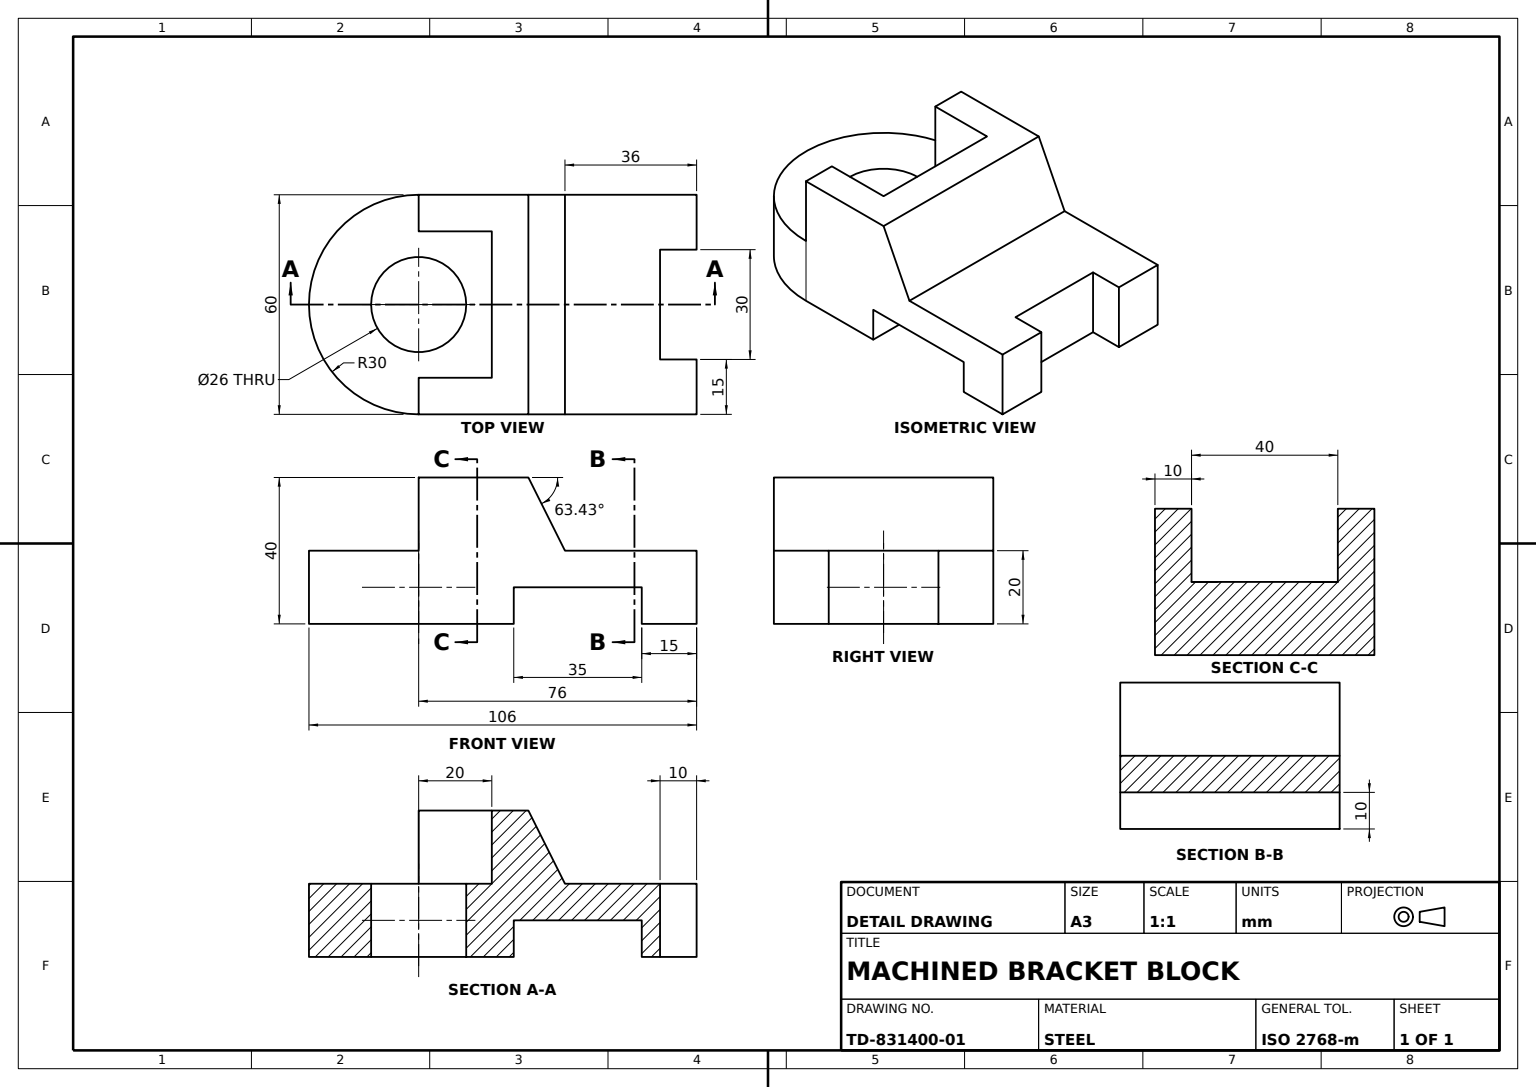
SolidWorks part; units mm, degrees
material "Plain Carbon Steel"
ref_plane "Front Plane" through (0, 0, 0) normal (0, 0, 1) x (1, 0, 0)
ref_plane "Top Plane" through (0, 0, 0) normal (0, 1, 0) x (1, 0, 0)
ref_plane "Right Plane" through (0, 0, 0) normal (1, 0, 0) x (0, 0, -1)
sketch "Base Plate Profile Sketch" plane through (0, 0, 0) normal (0, -1, 0) x (0, 0, -1)
  line L0 (0, 30) -> (76, 30)
  line L1 (76, 30) -> (76, -30)
  line L2 (76, -30) -> (0, -30)
  circle A0 centre (0, 0) radius 30
  circle A1 centre (0, 0) radius 13
  dimension "D1" = 30
  dimension "D2" = 26
  dimension "D3" = 76
extrude "Base Plate" add sketch "Base Plate Profile Sketch" against normal blind 20 contours L2 A0 L0 L1 | A0 A1
sketch "Base Slot Sketch" plane through (30, 0, 0) normal (1, 0, 0) x (0, 0, -1)
  line L0 (0, 0) -> (76, 0) construction
  line L2 (26, 0) -> (61, 0)
  line L3 (26, 0) -> (26, 10)
  line L4 (26, 10) -> (61, 10)
  line L5 (61, 0) -> (61, 10)
  line L6 (76, 20) -> (76, 0) construction
  dimension "D1" = 10
  dimension "D2" = 35
  dimension "D3" = 15
extrude "Base Slot Cut" cut sketch "Base Slot Sketch" against normal up to next
sketch "Bore Sketch" plane through (0, 20, 0) normal (0, 1, 0) x (1, 0, 0)
  line L0 (30, 76) -> (-30, 76) construction
  line L1 (-15, 76) -> (15, 76)
  line L2 (-15, 76) -> (-15, 66)
  line L3 (-15, 66) -> (15, 66)
  line L4 (15, 76) -> (15, 66)
  point P6 (0, 76)
  dimension "D1" = 10
  dimension "D2" = 30
extrude "Bore Cut" cut sketch "Bore Sketch" against normal up to next
sketch "Upright Block Profile Sketch" plane through (0, 0, 0) normal (1, 0, 0) x (0, 0, -1)
  line L0 (0, 20) -> (0, 40)
  line L1 (0, 40) -> (30, 40)
  line L2 (30, 40) -> (40, 20)
  line L3 (0, 20) -> (76, 20) construction
  line L4 (0, 20) -> (40, 20)
  line L5 (76, 20) -> (76, 0) construction
  dimension "D1" = 20
  dimension "D2" = 30
  dimension "D3" = 36
extrude "Upright Block" add sketch "Upright Block Profile Sketch" along normal through all and the other way through all
sketch "Upright Pocket Sketch" plane through (0, 40, 0) normal (0, 1, 0) x (1, 0, 0)
  line L0 (-13, 0) -> (-30, 0) construction
  line L1 (-20, 0) -> (20, 0)
  line L2 (-20, 0) -> (-20, 20)
  line L3 (-20, 20) -> (20, 20)
  line L4 (20, 0) -> (20, 20)
  point P6 (0, 0)
  dimension "D1" = 20
  dimension "D2" = 40
extrude "Upright Pocket Cut" cut sketch "Upright Pocket Sketch" against normal up to surface (20 mm away) up to face at (0, 20, -64.5)
